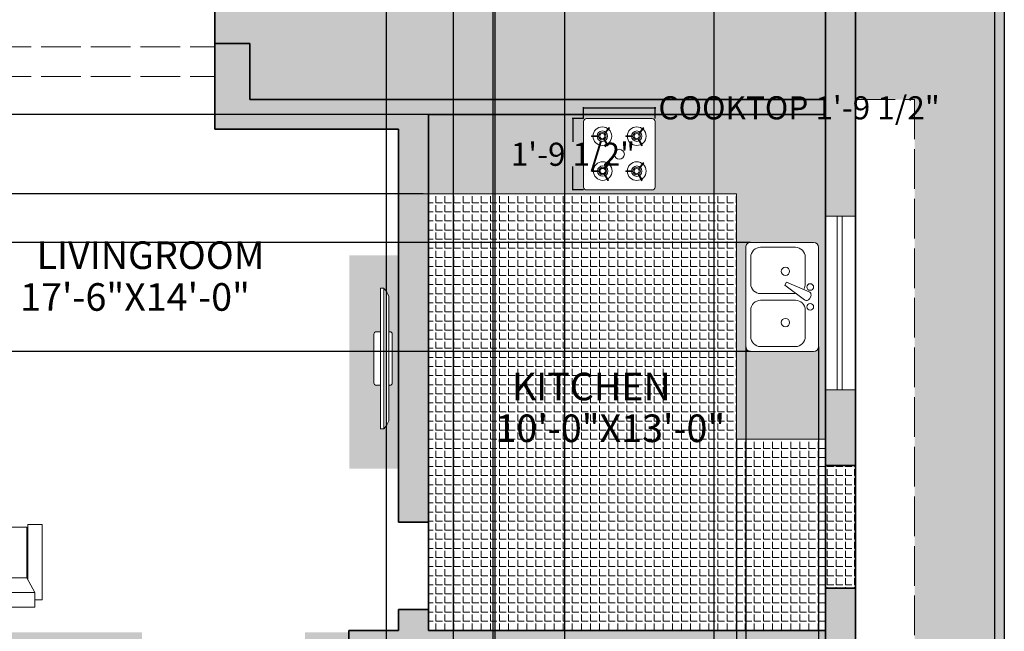
# Model space of a CAD drawing. Units: inches. Extents: x 1884 to 2398, y 474 to 1488.
# Tile 34 of 39: x 2099 to 2397, y 902 to 1087. Entities that reach past the tile are written whole.
import ezdxf

# ---------------------------------------------------------------- set-up
doc = ezdxf.new("R2010")
doc.units = ezdxf.units.IN
doc.header["$MEASUREMENT"] = 0
doc.linetypes.add('ACAD_ISO02W100', pattern=[15, 12, -3])
doc.layers.get('0').update_dxf_attribs({"color": 250})
for name, color, linetype, lineweight in [('A-ANNO-DIMS', 2, 'Continuous', 18), ('A-AREA-IDEN', 7, 'Continuous', 18), ('A-EQPM', 8, 'Continuous', 18), ('A-FLOR-CASE', 8, 'Continuous', 20), ('A-FLOR-FIXT', 8, 'Continuous', 18), ('A-FLOR-OVHD', 8, 'ACAD_ISO02W100', 18), ('A-FLOR-PATT', 254, 'Continuous', 13), ('A-WALL-PATT', 250, 'Continuous', 13), ('C-PROP', 7, 'Continuous', 30), ('furniture', 8, 'Continuous', 18), ('walls', 7, 'Continuous', 35), ('windows', 4, 'Continuous', 18)]:
    doc.layers.add(name, color=color, linetype=linetype, lineweight=lineweight)
doc.layers.add('A-FLOR-CASE-PATT', color=251, linetype='Continuous', lineweight=13, true_color=0x636466)
doc.layers.add('L-PVMT-PATT', color=9, linetype='Continuous', lineweight=13, true_color=0xc7c8ca)
doc.styles.add('ATT', font='TXT')
doc.styles.get("Standard").update_dxf_attribs({"font": 'arial.ttf'})
doc.dimstyles.get("Standard").update_dxf_attribs({"dimtxt": 7, "dimasz": 0.18, "dimexe": 0.18, "dimexo": 0.0625, "dimgap": 0.09, "dimtad": 0, "dimtih": 1, "dimtoh": 1, "dimzin": 0, "dimdsep": 46, "dimlunit": 3, "dimtxsty": 'Standard', "dimcen": 0.09, "dimadec": 0, "dimazin": 0, "dimtfac": 1, "dimtofl": 0, "dimtmove": 0, "dimatfit": 3, "dimfxl": 1, "dimtolj": 1, "dimtzin": 0, "dimarcsym": 0})

# ---------------------------------------------------------------- blocks, each defined once
blk = doc.blocks.new('15PSNK10')
at = {"color": 0, "linetype": 'ByBlock'}
for p, q in [((0, 15), (0, -15)), ((20.5, 16.5), (1.5, 16.5)), ((7, 15), (17.5, 15)), ((22, -15), (22, 15)), ((4, 4), (4, 12)), ((20.5, 12), (20.5, 4)), ((2.37, -0.1), (2.77, 0.6)), ((10.18, -3.57), (4.27, 0.87)), ((17.5, 1), (7, 1)), ((2.88, -1.54), (9.68, -4.43)), ((7.04, -1), (17.5, -1)), ((4, -12), (4, -4)), ((9.68, -4.43), (10.18, -3.57)), ((20.5, -4), (20.5, -12)), ((1.5, -16.5), (20.5, -16.5)), ((17.5, -15), (7, -15))]:
    blk.add_line(p, q, dxfattribs=at)
for centre, radius in [((10, 7.75), 1.25), ((2.5, 3), 1), ((2.5, -3), 1), ((10, -7.75), 1.25)]:
    blk.add_circle(centre, radius, dxfattribs=at)
for centre, radius, start, end in [((1.5, 15), 1.5, 90, 180), ((7, 12), 3, 90, 180), ((17.5, 12), 3, 0, 90), ((20.5, 15), 1.5, 0, 90), ((7, 4), 3, 180, 270), ((17.5, 4), 3, 270, 0), ((3.63, 0.1), 1, 50.5377, 150), ((3.23, -0.6), 1, 150, 249.4623), ((7, -4), 3, 146.607, 180), ((17.5, -4), 3, 0, 90), ((7, -12), 3, 180, 270), ((17.5, -12), 3, 270, 0), ((1.5, -15), 1.5, 180, 270), ((20.5, -15), 1.5, 270, 0)]:
    blk.add_arc(centre, radius, start, end, dxfattribs=at)
at = {"color": 0, "linetype": 'ByBlock', "style": 'ATT'}
for tag, p, flags in [('ITEM', (0, -26), 3), ('ROOM_NUMBER', (0, -35), 1)]:
    blk.add_attdef(tag, p, '', height=6, dxfattribs=dict(at, flags=flags))
blk = doc.blocks.new('4bstove')
at = {"layer": 'furniture'}
for p, q in [((1452.73, 1446.21), (1452.73, 1448.61)), ((1452.98, 1446.22), (1452.98, 1448.61)), ((1464.44, 1446.34), (1464.44, 1448.73)), ((1464.69, 1446.34), (1464.69, 1448.73)), ((1463.45, 1444.58), (1461.38, 1443.38)), ((1451.74, 1444.45), (1449.67, 1443.25)), ((1451.87, 1444.23), (1449.79, 1443.04)), ((1453.75, 1444.08), (1455.58, 1442.54)), ((1453.91, 1444.27), (1455.74, 1442.73)), ((1463.57, 1444.36), (1461.5, 1443.17)), ((1465.46, 1444.21), (1467.29, 1442.67)), ((1465.62, 1444.4), (1467.45, 1442.86)), ((1452.69, 1434.81), (1452.69, 1437.2)), ((1452.94, 1434.81), (1452.94, 1437.2)), ((1464.44, 1434.81), (1464.44, 1437.2)), ((1464.69, 1434.81), (1464.69, 1437.2)), ((1451.7, 1433.04), (1449.63, 1431.85)), ((1451.82, 1432.83), (1449.75, 1431.63)), ((1453.71, 1432.67), (1455.54, 1431.13)), ((1453.87, 1432.86), (1455.7, 1431.33)), ((1463.45, 1433.04), (1461.38, 1431.85)), ((1463.57, 1432.83), (1461.5, 1431.63)), ((1465.46, 1432.67), (1467.29, 1431.13)), ((1465.62, 1432.86), (1467.45, 1431.33))]:
    blk.add_line(p, q, dxfattribs=at)
for points in [[(1447.5, 1427.38), (1469.5, 1427.38, 0.414214), (1470.5, 1428.38), (1470.5, 1450.38, 0.414214), (1469.5, 1451.38), (1447.5, 1451.38, 0.414214), (1446.5, 1450.38), (1446.5, 1428.38, 0.414214)], [(1453.75, 1444.97, 1), (1452, 1444.97, 1)], [(1465.46, 1445.1, 1), (1463.71, 1445.1, 1)], [(1453.71, 1433.56, 1), (1451.96, 1433.56, 1)], [(1465.46, 1433.56, 1), (1463.71, 1433.56, 1)]]:
    blk.add_lwpolyline(points, format="xyb", close=True, dxfattribs=at)
for points in [[(1454.12, 1444.97, 1), (1451.62, 1444.97, 1), (1454.12, 1444.97, 1)], [(1465.83, 1445.1, 1), (1463.33, 1445.1, 1), (1465.83, 1445.1, 1)], [(1454.08, 1433.56, 1), (1451.58, 1433.56, 1), (1454.08, 1433.56, 1)], [(1465.83, 1433.56, 1), (1463.33, 1433.56, 1), (1465.83, 1433.56, 1)]]:
    blk.add_lwpolyline(points, format="xyb", dxfattribs=at)
for centre, radius in [((1452.87, 1444.97), 3.14), ((1464.58, 1445.1), 3.14), ((1452.87, 1444.97), 1.75), ((1464.58, 1445.1), 1.75), ((1458.5, 1439.38), 1.67), ((1452.83, 1433.56), 3.14), ((1452.83, 1433.56), 1.75), ((1464.58, 1433.56), 3.14), ((1464.58, 1433.56), 1.75)]:
    blk.add_circle(centre, radius, dxfattribs=at)
for centre, start, end in [((1452.87, 1444.97), 88.2645, 92.2039), ((1464.58, 1445.1), 88.2645, 92.2039), ((1452.87, 1444.97), 208.188, 212.1274), ((1452.87, 1444.97), 318.1018, 322.0412), ((1464.58, 1445.1), 208.188, 212.1274), ((1464.58, 1445.1), 318.1018, 322.0412), ((1452.83, 1433.56), 88.2645, 92.2039), ((1464.58, 1433.56), 88.2645, 92.2039)]:
    blk.add_arc(centre, 3.64, start, end, dxfattribs=at)
blk = doc.blocks.new('stove')
at = {"layer": 'furniture', "xscale": 0.9, "yscale": 0.9, "zscale": 0.9, "rotation": 89.99999999999999}
blk.add_blockref('4bstove', (1295.44, -1312.65), dxfattribs=at)
blk = doc.blocks.new('PLASMA-LARGE')
at = {"layer": 'furniture'}
for p, q in [((-7.26, 0), (7.26, 0)), ((-21, -2.5), (21, -2.5)), ((-21, -2.5), (-21, -3.5)), ((-18.61, -1), (18.61, -1)), ((-8, -1), (-8, -0.74)), ((8, -1), (8, -0.74)), ((21, -2.5), (21, -3.5)), ((-21, -3.5), (21, -3.5)), ((-8, -3.5), (-8, -4.76)), ((-7.26, -5.5), (7.26, -5.5)), ((8, -3.5), (8, -4.76))]:
    blk.add_line(p, q, dxfattribs=at)
for centre, radius, start, end in [((-7.26, -0.74), 0.744, 90, 180), ((7.26, -0.74), 0.744, 0, 90), ((-13.97, -11.05), 11.07, 114.7602, 129.4175), ((13.97, -11.05), 11.07, 50.5825, 65.2398), ((-7.26, -4.76), 0.744, 180, 270), ((7.26, -4.76), 0.744, 270, 0)]:
    blk.add_arc(centre, radius, start, end, dxfattribs=at)
blk = doc.blocks.new('FABRIC SOFA 1S')
at = {"layer": 'furniture'}
for p, q in [((3, 18.12), (34, 18.12)), ((3, 15.12), (3, 18.12)), ((34, 12.12), (34, 18.12)), ((0, -15.12), (0, 15.12)), ((6, 15.12), (0, 15.12)), ((6, -15.12), (6, 15.12)), ((12, 11.75), (6, 15.12)), ((11.33, 12.12), (34, 12.12)), ((6, -15.12), (12, -11.75)), ((11.33, -12.12), (34, -12.12)), ((34, -12.12), (34, -18.12)), ((6, -15.12), (0, -15.12)), ((3, -18.12), (3, -15.12)), ((3, -18.12), (34, -18.12))]:
    blk.add_line(p, q, dxfattribs=at)
blk.add_lwpolyline([(12, -11.75), (12, 11.75), (33, 11.75), (33, -11.75)], close=True, dxfattribs=at)
blk = doc.blocks.new('*D39')
at = {"layer": 'A-ANNO-DIMS', "color": 0, "lineweight": -2, "transparency": 16777216}
for p, q in [((2269.43, 1056.78), (2269.43, 1060.14)), ((2269.61, 1059.96), (2290.85, 1059.96)), ((2291.03, 1056.78), (2291.03, 1060.14)), ((2291.03, 1059.96), (2291.21, 1059.96))]:
    blk.add_line(p, q, dxfattribs=at)
at = {"layer": 'A-ANNO-DIMS', "color": 0, "lineweight": 100, "transparency": 16777216}
for points in [[(2269.61, 1059.99), (2269.61, 1059.93), (2269.43, 1059.96)], [(2290.85, 1059.99), (2290.85, 1059.93), (2291.03, 1059.96)]]:
    blk.add_solid(points, dxfattribs=at)
at = {"layer": 'Defpoints', "color": 0, "lineweight": 100, "transparency": 16777216}
for p in [(2291.03, 1059.96), (2269.43, 1056.72), (2291.03, 1056.72)]:
    blk.add_point(p, dxfattribs=at)
at = {"layer": 'A-ANNO-DIMS', "color": 0, "transparency": 16777216, "insert": (2334.53, 1059.96), "char_height": 7, "attachment_point": 5}
blk.add_mtext('\\A1;COOKTOP 1\'-9 1/2"', dxfattribs=at)
blk = doc.blocks.new('*D40')
at = {"layer": 'A-ANNO-DIMS', "color": 0, "lineweight": -2, "transparency": 16777216}
for p, q in [((2269.37, 1056.72), (2266.01, 1056.72)), ((2266.19, 1056.54), (2266.19, 1049.63)), ((2266.19, 1035.3), (2266.19, 1042.21)), ((2269.37, 1035.12), (2266.01, 1035.12))]:
    blk.add_line(p, q, dxfattribs=at)
at = {"layer": 'A-ANNO-DIMS', "color": 0, "lineweight": 100, "transparency": 16777216}
for points in [[(2266.16, 1056.54), (2266.22, 1056.54), (2266.19, 1056.72)], [(2266.16, 1035.3), (2266.22, 1035.3), (2266.19, 1035.12)]]:
    blk.add_solid(points, dxfattribs=at)
at = {"layer": 'Defpoints', "color": 0, "lineweight": 100, "transparency": 16777216}
for p in [(2266.19, 1056.72), (2269.43, 1056.72), (2269.43, 1035.12)]:
    blk.add_point(p, dxfattribs=at)
at = {"layer": 'A-ANNO-DIMS', "color": 0, "transparency": 16777216, "insert": (2266.19, 1045.92), "char_height": 7, "attachment_point": 5}
blk.add_mtext('\\A1;1\'-9 1/2"', dxfattribs=at)
blk = doc.blocks.new('*D44')
at = {"layer": 'A-ANNO-DIMS', "color": 0, "lineweight": -2, "transparency": 16777216}
for p, q in [((2209.76, 1247.82), (2209.76, 484)), ((2230.03, 1247.82), (2230.03, 484)), ((2209.94, 484.18), (2229.85, 484.18)), ((2230.03, 484.18), (2230.21, 484.18))]:
    blk.add_line(p, q, dxfattribs=at)
at = {"layer": 'A-ANNO-DIMS', "color": 0, "lineweight": 100, "transparency": 16777216}
for points in [[(2209.94, 484.21), (2209.94, 484.15), (2209.76, 484.18)], [(2229.85, 484.21), (2229.85, 484.15), (2230.03, 484.18)]]:
    blk.add_solid(points, dxfattribs=at)
at = {"layer": 'Defpoints', "color": 0, "lineweight": 100, "transparency": 16777216}
for p in [(2209.76, 1247.88), (2230.03, 1247.88), (2230.03, 484.18)]:
    blk.add_point(p, dxfattribs=at)
at = {"layer": 'A-ANNO-DIMS', "color": 0, "transparency": 16777216, "insert": (2247.43, 484.18), "char_height": 7, "attachment_point": 5}
blk.add_mtext('\\A1;1\'-8 1/2"', dxfattribs=at)
blk = doc.blocks.new('*D45')
at = {"layer": 'A-ANNO-DIMS', "color": 0, "lineweight": -2, "transparency": 16777216}
for p, q in [((2242.62, 1322.82), (2242.62, 484)), ((2263.62, 1322.82), (2263.62, 484)), ((2242.8, 484.18), (2244.05, 484.18)), ((2263.44, 484.18), (2262.18, 484.18))]:
    blk.add_line(p, q, dxfattribs=at)
at = {"layer": 'A-ANNO-DIMS', "color": 0, "lineweight": 100, "transparency": 16777216}
for points in [[(2242.8, 484.21), (2242.8, 484.15), (2242.62, 484.18)], [(2263.44, 484.21), (2263.44, 484.15), (2263.62, 484.18)]]:
    blk.add_solid(points, dxfattribs=at)
at = {"layer": 'Defpoints', "color": 0, "lineweight": 100, "transparency": 16777216}
for p in [(2242.62, 1322.88), (2263.62, 1322.88), (2263.62, 484.18)]:
    blk.add_point(p, dxfattribs=at)
at = {"layer": 'A-ANNO-DIMS', "color": 0, "transparency": 16777216, "insert": (2253.12, 484.18), "char_height": 7, "attachment_point": 5}
blk.add_mtext('\\A1;1\'-9"', dxfattribs=at)
blk = doc.blocks.new('*D47')
at = {"layer": 'A-ANNO-DIMS', "color": 0, "lineweight": -2, "transparency": 16777216}
for p, q in [((2315.59, 959.7), (2315.59, 484)), ((2342.53, 959.7), (2342.53, 484)), ((2315.77, 484.18), (2319.61, 484.18)), ((2342.35, 484.18), (2338.51, 484.18))]:
    blk.add_line(p, q, dxfattribs=at)
at = {"layer": 'A-ANNO-DIMS', "color": 0, "lineweight": 100, "transparency": 16777216}
for points in [[(2315.77, 484.21), (2315.77, 484.15), (2315.59, 484.18)], [(2342.35, 484.21), (2342.35, 484.15), (2342.53, 484.18)]]:
    blk.add_solid(points, dxfattribs=at)
at = {"layer": 'Defpoints', "color": 0, "lineweight": 100, "transparency": 16777216}
for p in [(2315.59, 959.77), (2342.53, 959.77), (2342.53, 484.18)]:
    blk.add_point(p, dxfattribs=at)
at = {"layer": 'A-ANNO-DIMS', "color": 0, "transparency": 16777216, "insert": (2329.06, 484.18), "char_height": 7, "attachment_point": 5}
blk.add_mtext('\\A1;2\'-3"', dxfattribs=at)
blk = doc.blocks.new('*D48')
at = {"layer": 'A-ANNO-DIMS', "color": 0, "lineweight": -2, "transparency": 16777216}
for p, q in [((2222.47, 1057.97), (1902.43, 1057.97)), ((1902.61, 1057.79), (1902.61, 1049.64)), ((1902.61, 1034.16), (1902.61, 1042.31)), ((2220.98, 1033.98), (1902.43, 1033.98))]:
    blk.add_line(p, q, dxfattribs=at)
at = {"layer": 'A-ANNO-DIMS', "color": 0, "lineweight": 100, "transparency": 16777216}
for points in [[(1902.58, 1057.79), (1902.64, 1057.79), (1902.61, 1057.97)], [(1902.58, 1034.16), (1902.64, 1034.16), (1902.61, 1033.98)]]:
    blk.add_solid(points, dxfattribs=at)
at = {"layer": 'Defpoints', "color": 0, "lineweight": 100, "transparency": 16777216}
for p in [(1902.61, 1057.97), (2222.53, 1057.97), (2221.05, 1033.98)]:
    blk.add_point(p, dxfattribs=at)
at = {"layer": 'A-ANNO-DIMS', "color": 0, "transparency": 16777216, "insert": (1902.61, 1045.97), "char_height": 7, "attachment_point": 5}
blk.add_mtext('\\A1;2\'-0"', dxfattribs=at)
blk = doc.blocks.new('*D49')
at = {"layer": 'A-ANNO-DIMS', "color": 0, "lineweight": -2, "transparency": 16777216}
for p, q in [((2318.41, 987.72), (2318.41, 484)), ((2340.41, 987.72), (2340.41, 484)), ((2318.59, 484.18), (2340.23, 484.18)), ((2340.41, 484.18), (2340.59, 484.18))]:
    blk.add_line(p, q, dxfattribs=at)
at = {"layer": 'A-ANNO-DIMS', "color": 0, "lineweight": 100, "transparency": 16777216}
for points in [[(2318.59, 484.21), (2318.59, 484.15), (2318.41, 484.18)], [(2340.23, 484.21), (2340.23, 484.15), (2340.41, 484.18)]]:
    blk.add_solid(points, dxfattribs=at)
at = {"layer": 'Defpoints', "color": 0, "lineweight": 100, "transparency": 16777216}
for p in [(2318.41, 987.78), (2340.41, 987.78), (2340.41, 484.18)]:
    blk.add_point(p, dxfattribs=at)
at = {"layer": 'A-ANNO-DIMS', "color": 0, "transparency": 16777216, "insert": (2352.37, 484.18), "char_height": 7, "attachment_point": 5}
blk.add_mtext('\\A1;1\'-10"', dxfattribs=at)
blk = doc.blocks.new('*D50')
at = {"layer": 'A-ANNO-DIMS', "color": 0, "lineweight": -2, "transparency": 16777216}
for p, q in [((2319.85, 1019.28), (1902.43, 1019.28)), ((1902.61, 1019.1), (1902.61, 1006.44)), ((1902.61, 986.46), (1902.61, 999.11)), ((2319.85, 986.28), (1902.43, 986.28))]:
    blk.add_line(p, q, dxfattribs=at)
at = {"layer": 'A-ANNO-DIMS', "color": 0, "lineweight": 100, "transparency": 16777216}
for points in [[(1902.58, 1019.1), (1902.64, 1019.1), (1902.61, 1019.28)], [(1902.58, 986.46), (1902.64, 986.46), (1902.61, 986.28)]]:
    blk.add_solid(points, dxfattribs=at)
at = {"layer": 'Defpoints', "color": 0, "lineweight": 100, "transparency": 16777216}
for p in [(1902.61, 1019.28), (2319.91, 1019.28), (2319.91, 986.28)]:
    blk.add_point(p, dxfattribs=at)
at = {"layer": 'A-ANNO-DIMS', "color": 0, "transparency": 16777216, "insert": (1902.61, 1002.78), "char_height": 7, "attachment_point": 5}
blk.add_mtext('\\A1;2\'-9"', dxfattribs=at)
blk = doc.blocks.new('*D52')
at = {"layer": 'A-ANNO-DIMS', "color": 0, "lineweight": -2, "transparency": 16777216}
for p, q in [((2308.85, 820.89), (2308.85, 1477.76)), ((2309.03, 1477.58), (2342.35, 1477.58)), ((2342.53, 820.89), (2342.53, 1477.76)), ((2342.53, 1477.58), (2342.71, 1477.58))]:
    blk.add_line(p, q, dxfattribs=at)
at = {"layer": 'A-ANNO-DIMS', "color": 0, "lineweight": 100, "transparency": 16777216}
for points in [[(2309.03, 1477.61), (2309.03, 1477.55), (2308.85, 1477.58)], [(2342.35, 1477.61), (2342.35, 1477.55), (2342.53, 1477.58)]]:
    blk.add_solid(points, dxfattribs=at)
at = {"layer": 'Defpoints', "color": 0, "lineweight": 100, "transparency": 16777216}
for p in [(2342.53, 1477.58), (2308.85, 820.83), (2342.53, 820.83)]:
    blk.add_point(p, dxfattribs=at)
at = {"layer": 'A-ANNO-DIMS', "color": 0, "transparency": 16777216, "insert": (2360.32, 1477.58), "char_height": 7, "attachment_point": 5}
blk.add_mtext('\\A1;2\'-9 1/2"', dxfattribs=at)
blk = doc.blocks.new('*D54')
at = {"layer": 'A-ANNO-DIMS', "color": 0, "lineweight": -2, "transparency": 16777216}
for p, q in [((2242.06, 893.03), (2242.06, 1477.76)), ((2242.24, 1477.58), (2266.06, 1477.58)), ((2308.67, 1477.58), (2284.85, 1477.58)), ((2308.85, 893.03), (2308.85, 1477.76))]:
    blk.add_line(p, q, dxfattribs=at)
at = {"layer": 'A-ANNO-DIMS', "color": 0, "lineweight": 100, "transparency": 16777216}
for points in [[(2242.24, 1477.61), (2242.24, 1477.55), (2242.06, 1477.58)], [(2308.67, 1477.61), (2308.67, 1477.55), (2308.85, 1477.58)]]:
    blk.add_solid(points, dxfattribs=at)
at = {"layer": 'Defpoints', "color": 0, "lineweight": 100, "transparency": 16777216}
for p in [(2308.85, 1477.58), (2242.06, 892.97), (2308.85, 892.97)]:
    blk.add_point(p, dxfattribs=at)
at = {"layer": 'A-ANNO-DIMS', "color": 0, "transparency": 16777216, "insert": (2275.45, 1477.58), "char_height": 7, "attachment_point": 5}
blk.add_mtext('\\A1;5\'-7"', dxfattribs=at)

msp = doc.modelspace()

# ---------------------------------------------------------------- hatches: boundary and pattern name
at = {"layer": 'A-FLOR-CASE-PATT'}
h = msp.add_hatch(color=256, dxfattribs=at)
h.dxf.hatch_style = 1
h.paths.add_polyline_path([(2342.529, 1057.966), (2222.529, 1057.966), (2222.529, 1033.976), (2315.591, 1033.976), (2315.591, 959.766), (2342.529, 959.766)])
h.paths.add_polyline_path([(2269.433, 1055.817, -0.4142136), (2270.333, 1056.717), (2290.133, 1056.717, -0.4142136), (2291.033, 1055.817), (2291.033, 1036.017, -0.4142136), (2290.133, 1035.117), (2270.333, 1035.117, -0.4142136), (2269.433, 1036.017)], flags=16)
h.paths.add_polyline_path([(2271.815, 1051.262, -0.0171907), (2271.814, 1051.487), (2272.265, 1051.487, -0.6105283), (2276.81, 1053.623), (2277.099, 1053.968, -0.0171906), (2277.272, 1053.824), (2276.982, 1053.479, -0.2116406), (2277.909, 1051.388, -0.2564461), (2276.601, 1049.006), (2276.827, 1048.616, -0.0171907), (2276.632, 1048.503), (2276.407, 1048.893, -0.5505708), (2272.266, 1051.262)], flags=0)
h.paths.add_polyline_path([(2271.929, 1040.951), (2272.379, 1040.951, -0.6105283), (2276.925, 1043.087), (2277.214, 1043.432, -0.0171906), (2277.387, 1043.288), (2277.097, 1042.943, -0.2116406), (2278.024, 1040.852, -0.2564461), (2276.716, 1038.47), (2276.941, 1038.08, -0.0171907), (2276.747, 1037.967), (2276.522, 1038.357, -0.5505708), (2272.38, 1040.726), (2271.93, 1040.726, -0.0171907)], flags=0)
h.paths.add_polyline_path([(2276.661, 1051.388, -1), (2273.511, 1051.388, -1)], flags=0)
h.paths.add_polyline_path([(2275.086, 1052.513, -1), (2275.086, 1050.263, -1)], flags=0)
h.paths.add_polyline_path([(2275.086, 1052.175, -1), (2275.086, 1050.6, -1)], flags=0)
h.paths.add_polyline_path([(2276.776, 1040.852, -1), (2273.626, 1040.852, -1)], flags=0)
h.paths.add_polyline_path([(2275.201, 1041.977, -1), (2275.201, 1039.727, -1)], flags=0)
h.paths.add_polyline_path([(2275.201, 1041.639, -1), (2275.201, 1040.064, -1)], flags=0)
h.paths.add_polyline_path([(2281.737, 1045.917, -1), (2278.73, 1045.917, -1)], flags=0)
h.paths.add_polyline_path([(2282.197, 1051.262, -0.0171907), (2282.196, 1051.487), (2282.647, 1051.487, -0.9825922), (2288.291, 1051.388, -0.9779445), (2282.648, 1051.262)], flags=0)
h.paths.add_polyline_path([(2282.196, 1040.912), (2282.647, 1040.912, -0.9825922), (2288.291, 1040.813, -0.9779445), (2282.648, 1040.687), (2282.197, 1040.687, -0.0171907)], flags=0)
h.paths.add_polyline_path([(2287.043, 1051.388, -1), (2283.893, 1051.388, -1)], flags=0)
h.paths.add_polyline_path([(2285.468, 1052.513, -1), (2285.468, 1050.263, -1)], flags=0)
h.paths.add_polyline_path([(2285.468, 1052.175, -1), (2285.468, 1050.6, -1)], flags=0)
h.paths.add_polyline_path([(2287.043, 1040.813, -1), (2283.893, 1040.813, -1)], flags=0)
h.paths.add_polyline_path([(2285.468, 1041.938, -1), (2285.468, 1039.688, -1)], flags=0)
h.paths.add_polyline_path([(2285.468, 1041.601, -1), (2285.468, 1040.026, -1)], flags=0)
h.paths.add_polyline_path([(2319.909, 1019.278), (2338.909, 1019.278, -0.4142136), (2340.409, 1017.778), (2340.409, 987.778, -0.4142136), (2338.909, 986.278), (2319.909, 986.278, -0.4142136), (2318.409, 987.778), (2318.409, 1017.778, -0.4142136)], flags=16)
h.paths.add_polyline_path([(2337.528, 1004.314, -0.4631995), (2338.044, 1002.878), (2337.641, 1002.18, -0.4369422), (2336.21, 1001.854), (2330.231, 1006.345), (2330.731, 1007.211)], flags=0)
h.paths.add_polyline_path([(2322.909, 1001.778), (2333.409, 1001.778, -0.4142136), (2336.409, 998.778), (2336.409, 990.778, -0.4142136), (2333.409, 987.778), (2322.909, 987.778, -0.4142136), (2319.909, 990.778), (2319.909, 998.778, -0.4142136)], flags=0)
h.paths.add_polyline_path([(2331.659, 1010.528, -1), (2329.159, 1010.528, -1)], flags=0)
h.paths.add_polyline_path([(2331.659, 995.028, -1), (2329.159, 995.028, -1)], flags=0)
h.paths.add_polyline_path([(2338.909, 1005.778, -1), (2336.909, 1005.778, -1)], flags=0)
h.paths.add_polyline_path([(2338.909, 999.778, -1), (2336.909, 999.778, -1)], flags=0)
h = msp.add_hatch(color=256, dxfattribs=at)
h.dxf.hatch_style = 1
h.paths.add_polyline_path([(2198.68, 1015.326), (2213.576, 1015.326), (2213.576, 950.883), (2198.68, 950.883)])
h.paths.add_polyline_path([(2208.087, 962.907), (2209.098, 962.907, 0.0640419), (2210.615, 965.326), (2210.615, 976.054), (2210.874, 976.054, 0.4142136), (2211.626, 976.807), (2211.626, 991.482, 0.4142136), (2210.874, 992.235), (2210.615, 992.235), (2210.615, 1002.962, 0.0640419), (2209.098, 1005.381), (2208.087, 1005.381), (2208.087, 992.235), (2206.817, 992.235, 0.4142136), (2206.064, 991.482), (2206.064, 976.807, 0.4142136), (2206.817, 976.054), (2208.087, 976.054)], flags=16)
at = {"layer": 'A-FLOR-PATT'}
h = msp.add_hatch(color=256, dxfattribs=at)
h.dxf.hatch_style = 1
h.paths.add_polyline_path([(2117.529, 815.801), (2126.529, 815.801), (2126.529, 880.382), (2117.529, 880.382), (2117.529, 892.385), (1961.529, 892.385), (1961.529, 756.915), (1964.529, 756.915), (1964.529, 759.915), (1995.529, 759.915), (1995.529, 753.915), (1972.862, 753.915), (1967.529, 756.915), (1967.529, 654.915), (1972.862, 657.915), (1995.529, 657.915), (1995.529, 651.915), (1964.529, 651.915), (1964.529, 654.915), (1961.529, 654.915), (1961.529, 640.385), (2117.529, 640.385), (2117.529, 646.578), (2126.529, 646.578), (2126.529, 676.183), (2117.529, 676.183)])
h.paths.add_polyline_path([(2012.246, 808.929), (2012.05, 810.185), (2032.542, 810.185), (2032.346, 808.929)], flags=16)
h.paths.add_polyline_path([(2010.381, 820.864), (1994.658, 820.864), (1994.658, 831.561), (1984.608, 833.132), (1984.608, 853.821), (1994.658, 855.391), (1994.658, 866.089), (2010.381, 866.089), (2011.951, 876.139), (2032.64, 876.139), (2034.211, 866.089), (2045.556, 866.089), (2047.127, 876.139), (2067.816, 876.139), (2069.386, 866.089), (2085.109, 866.089), (2085.109, 855.391), (2095.159, 853.821), (2095.159, 833.132), (2085.109, 831.561), (2085.109, 820.864), (2069.386, 820.864), (2067.816, 810.814), (2047.127, 810.814), (2045.556, 820.864), (2034.211, 820.864), (2032.64, 810.814), (2011.951, 810.814)], flags=16)
h.paths.add_polyline_path([(1982.724, 833.426), (1982.724, 853.526), (1983.98, 853.723), (1983.98, 833.23)], flags=16)
h.paths.add_polyline_path([(1994.529, 753.54), (1994.529, 658.29), (1973.529, 658.29), (1973.529, 753.54)], flags=16)
h.paths.add_polyline_path([(2084.486, 843.527), (2084.592, 843.502), (2084.681, 843.487), (2084.813, 843.477), (2084.913, 843.477), (2084.669, 843.482), (2084.336, 843.565), (2084.116, 843.617), (2083.8, 843.686), (2083.105, 843.827), (2082.836, 843.874), (2083.604, 843.729), (2084.206, 843.597)], flags=0)
h.paths.add_polyline_path([(2047.421, 808.929), (2047.225, 810.185), (2067.718, 810.185), (2067.521, 808.929)], flags=16)
h.paths.add_polyline_path([(2066.01, 849.505), (2066.429, 849.687), (2066.798, 849.882), (2067.129, 850.085), (2067.43, 850.293), (2067.711, 850.502), (2068.176, 850.856), (2068.689, 851.205), (2069.305, 851.531), (2070.015, 851.784), (2070.844, 851.944), (2071.081, 851.956), (2070.629, 851.902), (2070.212, 851.822), (2069.827, 851.717), (2069.471, 851.59), (2069.139, 851.443), (2068.828, 851.279), (2068.534, 851.1), (2068.254, 850.909), (2067.983, 850.709), (2067.502, 850.343), (2066.951, 849.962), (2066.224, 849.579)], flags=0)
h.paths.add_polyline_path([(2059.423, 853.221), (2059.827, 853.278), (2060.171, 853.358), (2060.465, 853.463), (2060.714, 853.589), (2060.926, 853.736), (2061.107, 853.902), (2061.258, 854.086), (2061.377, 854.284), (2061.462, 854.495), (2061.514, 854.715), (2061.53, 854.943), (2061.508, 855.176), (2061.449, 855.411), (2061.352, 855.646), (2061.224, 855.882), (2061.07, 856.117), (2060.9, 856.353), (2060.719, 856.588), (2060.406, 856.993), (2060.103, 857.424), (2059.858, 857.888), (2059.691, 858.467), (2059.836, 859.091), (2060.305, 859.532), (2060.844, 859.798), (2061.513, 859.935), (2062.253, 859.905), (2062.483, 859.849), (2062.078, 859.912), (2061.695, 859.928), (2061.336, 859.899), (2061.005, 859.831), (2060.703, 859.729), (2060.437, 859.597), (2060.208, 859.441), (2060.021, 859.265), (2059.879, 859.075), (2059.785, 858.874), (2059.737, 858.664), (2059.73, 858.447), (2059.761, 858.224), (2059.827, 857.996), (2059.923, 857.765), (2060.047, 857.53), (2060.193, 857.295), (2060.359, 857.06), (2060.537, 856.824), (2060.867, 856.399), (2061.171, 855.978), (2061.422, 855.518), (2061.567, 854.943), (2061.41, 854.272), (2060.947, 853.707), (2060.335, 853.397), (2059.649, 853.236)], flags=0)
h.paths.add_polyline_path([(2050.778, 859.745), (2051.07, 859.87), (2051.295, 860.017), (2051.467, 860.183), (2051.594, 860.365), (2051.679, 860.56), (2051.726, 860.763), (2051.739, 860.971), (2051.722, 861.18), (2051.677, 861.387), (2051.609, 861.587), (2051.521, 861.779), (2051.421, 861.962), (2051.312, 862.138), (2051.203, 862.307), (2050.966, 862.68), (2050.793, 863.193), (2051.021, 863.699), (2051.483, 864.018), (2052.09, 864.138), (2052.773, 864.157), (2053.007, 864.142), (2052.603, 864.152), (2052.258, 864.142), (2051.965, 864.113), (2051.716, 864.064), (2051.504, 863.995), (2051.322, 863.907), (2051.17, 863.802), (2051.048, 863.682), (2050.954, 863.55), (2050.891, 863.408), (2050.856, 863.259), (2050.851, 863.105), (2050.876, 862.948), (2050.929, 862.791), (2051.005, 862.633), (2051.098, 862.472), (2051.203, 862.307), (2051.312, 862.138), (2051.556, 861.742), (2051.751, 861.167), (2051.712, 860.535), (2051.398, 860.085), (2050.949, 859.79)], flags=0)
h.paths.add_polyline_path([(2022.768, 719.264), (2050.461, 719.264), (2050.461, 717.226), (2052.426, 717.226), (2052.426, 715.033), (2050.461, 715.033), (2050.461, 703.738), (2022.768, 703.738)], flags=16)
h.paths.add_polyline_path([(2012.246, 878.023), (2032.346, 878.023), (2032.542, 876.767), (2012.05, 876.767)], flags=16)
h.paths.add_polyline_path([(2035.324, 713.103), (2035.342, 713.294), (2035.192, 713.202)], flags=0)
h.paths.add_polyline_path([(2036.484, 711.63), (2036.583, 711.849), (2036.39, 711.898)], flags=0)
h.paths.add_polyline_path([(2036.074, 712.744), (2035.993, 712.481), (2035.724, 712.516), (2035.794, 712.726)], flags=0)
h.paths.add_polyline_path([(2035.846, 710.909), (2035.753, 710.958), (2035.702, 710.88)], flags=0)
h.paths.add_polyline_path([(2037.818, 712.019), (2037.948, 712.06), (2037.987, 712.161), (2037.815, 712.02)], flags=0)
h.paths.add_polyline_path([(2038.451, 709.517), (2038.464, 709.428), (2038.586, 709.442)], flags=0)
h.paths.add_polyline_path([(2037.805, 709.806), (2037.818, 709.807), (2037.804, 709.823)], flags=0)
h.paths.add_polyline_path([(2036.7, 711.245), (2036.698, 711.236), (2036.813, 711.211)], flags=0)
h.paths.add_polyline_path([(2035.928, 708.897), (2035.668, 708.871), (2035.706, 708.667)], flags=0)
h.paths.add_polyline_path([(2036.414, 710.976), (2035.932, 709.859), (2036.792, 710.484), (2036.5, 710.934)], flags=0)
h.paths.add_polyline_path([(2038.298, 712.115), (2038.499, 712.058), (2038.612, 712.269), (2038.39, 712.332)], flags=0)
h.paths.add_polyline_path([(2047.421, 878.023), (2067.521, 878.023), (2067.718, 876.767), (2047.225, 876.767)], flags=16)
h.paths.add_polyline_path([(2049.647, 705.093, -1), (2048.845, 705.093, -1)], flags=0)
h.paths.add_polyline_path([(2095.787, 853.723), (2097.043, 853.526), (2097.043, 833.426), (2095.787, 833.23)], flags=16)
h.paths.add_polyline_path([(2110.739, 745.339), (2111.75, 745.339, -0.0640419), (2113.267, 742.92), (2113.267, 732.192), (2113.526, 732.192, -0.4142136), (2114.278, 731.439), (2114.278, 716.764, -0.4142136), (2113.526, 716.011), (2113.267, 716.011), (2113.267, 705.284, -0.0640419), (2111.75, 702.864), (2110.739, 702.864), (2110.739, 716.011), (2109.469, 716.011, -0.4142136), (2108.716, 716.764), (2108.716, 731.439, -0.4142136), (2109.469, 732.192), (2110.739, 732.192)], flags=16)
h.paths.add_polyline_path([(1998.045, 668.909), (2002.449, 668.909), (2002.449, 652.273), (2002.724, 652.763), (2002.724, 668.175), (2019.972, 668.175), (2019.972, 652.763), (2020.247, 652.273), (2020.247, 668.909), (2024.651, 668.909), (2029.055, 668.909), (2029.055, 652.273), (2029.33, 652.763), (2029.33, 668.175), (2046.578, 668.175), (2046.578, 652.763), (2046.853, 652.273), (2046.853, 668.909), (2051.257, 668.909), (2051.257, 646.157), (2049.055, 646.157), (2049.055, 643.955), (2026.853, 643.955), (2026.853, 646.157), (2024.651, 646.157), (2022.449, 646.157), (2022.449, 643.955), (2000.247, 643.955), (2000.247, 646.157), (1998.045, 646.157)], flags=16)
h.paths.add_polyline_path([(2342.529, 1247.885), (2265.892, 1247.885), (2230.029, 1247.885), (2209.755, 1247.885), (2168.6, 1247.885), (2168.6, 1104.929), (2158.029, 1104.929), (2158.029, 1079.411), (2168.6, 1079.411), (2168.6, 1062.466), (2342.529, 1062.466), (2342.529, 1093.809)])
h.paths.add_polyline_path([(2215.03, 1153.876), (2215.03, 1164.739), (2187.559, 1164.739), (2187.442, 1152.641), (2173.568, 1152.641), (2173.684, 1164.739), (2173.684, 1218.739), (2173.801, 1230.837), (2187.675, 1230.837), (2187.559, 1218.739), (2215.03, 1218.739), (2215.03, 1225.879), (2245.053, 1225.879), (2245.053, 1153.876)], flags=16)
h.paths.add_polyline_path([(2192.147, 1164.797), (2184.963, 1174.54), (2184.915, 1174.54), (2176.755, 1174.54), (2176.755, 1190.363), (2184.915, 1190.363), (2184.915, 1196.819), (2176.755, 1196.819), (2176.755, 1212.641), (2184.915, 1212.641), (2184.915, 1174.606), (2184.963, 1174.54), (2192.147, 1174.54)], flags=0)
h.paths.add_polyline_path([(2184.971, 1158.364, -1), (2176.039, 1158.364, -1)], flags=0)
h.paths.add_polyline_path([(2335.555, 1161.985), (2335.555, 1175.132), (2334.285, 1175.132, -0.4142136), (2333.533, 1175.885), (2333.533, 1190.56, -0.4142136), (2334.285, 1191.313), (2335.555, 1191.313), (2335.555, 1204.46), (2336.567, 1204.46, -0.0640419), (2338.083, 1202.04), (2338.083, 1191.313), (2338.342, 1191.313, -0.4142136), (2339.095, 1190.56), (2339.095, 1175.885, -0.4142136), (2338.342, 1175.132), (2338.083, 1175.132), (2338.083, 1164.405, -0.0640419), (2336.567, 1161.985)], flags=16)
h.paths.add_polyline_path([(2176.155, 1224.462, -1), (2185.087, 1224.462, -1)], flags=0)
h.paths.add_polyline_path([(2158.029, 1276.197), (2158.029, 1322.885), (2148.233, 1322.885), (2092.029, 1322.885), (1961.529, 1322.885), (1961.529, 1166.885), (2116.005, 1166.885), (2116.005, 1157.885), (2152.638, 1157.885), (2152.638, 1166.885), (2158.029, 1166.885)])
h.paths.add_polyline_path([(2006.352, 1204.245), (2006.352, 1215.108), (1978.881, 1215.108), (1978.764, 1203.01), (1964.89, 1203.01), (1965.006, 1215.108), (1965.006, 1269.108), (1965.123, 1281.207), (1978.997, 1281.207), (1978.881, 1269.108), (2006.352, 1269.108), (2006.352, 1276.248), (2036.375, 1276.248), (2036.375, 1204.245)], flags=16)
h.paths.add_polyline_path([(1983.469, 1215.166), (1976.285, 1224.909), (1976.237, 1224.909), (1968.077, 1224.909), (1968.077, 1240.732), (1976.237, 1240.732), (1976.237, 1247.188), (1968.077, 1247.188), (1968.077, 1263.011), (1976.237, 1263.011), (1976.237, 1224.975), (1976.285, 1224.909), (1983.469, 1224.909)], flags=0)
h.paths.add_polyline_path([(1976.293, 1208.733, -1), (1967.361, 1208.733, -1)], flags=0)
h.paths.add_polyline_path([(1967.477, 1274.832, -1), (1976.41, 1274.832, -1)], flags=0)
h.paths.add_polyline_path([(2152.587, 1223.485), (2152.587, 1236.632), (2151.317, 1236.632, -0.4142136), (2150.564, 1237.385), (2150.564, 1252.06, -0.4142136), (2151.317, 1252.813), (2152.587, 1252.813), (2152.587, 1265.959), (2153.598, 1265.959, -0.0640419), (2155.115, 1263.54), (2155.115, 1252.813), (2155.374, 1252.813, -0.4142136), (2156.126, 1252.06), (2156.126, 1237.385, -0.4142136), (2155.374, 1236.632), (2155.115, 1236.632), (2155.115, 1225.904, -0.0640419), (2153.598, 1223.485)], flags=16)
h.paths.add_polyline_path([(2250.676, 1161.101), (2322.077, 1161.101), (2322.077, 1173.886), (2250.676, 1173.886)], flags=24)
h.paths.add_polyline_path([(2255.61, 1173.712), (2320.136, 1173.712), (2320.136, 1186.659), (2255.61, 1186.659)], flags=24)
h.paths.add_polyline_path([(2053.687, 1230.837), (2125.089, 1230.837), (2125.089, 1243.622), (2053.687, 1243.622)], flags=24)
h.paths.add_polyline_path([(2058.622, 1243.448), (2123.147, 1243.448), (2123.147, 1256.395), (2058.622, 1256.395)], flags=24)
h = msp.add_hatch(dxfattribs=at)
h.set_pattern_fill('ANGLE', color=256, scale=10)
h.set_pattern_definition([(0, (0, 0), (0, 2.75), [2, -0.75]), (90, (0, 0), (-2.75, 2e-16), [2, -0.75])])
h.paths.add_polyline_path([(2315.591, 1033.976), (2222.529, 1033.976), (2222.529, 934.675), (2222.529, 901.966), (2342.529, 901.966), (2342.529, 914.773), (2351.529, 914.773), (2351.529, 951.86), (2342.529, 951.86), (2342.529, 959.766), (2315.591, 959.766)])
at = {"layer": 'A-WALL-PATT'}
h = msp.add_hatch(color=256, dxfattribs=at)
h.dxf.hatch_style = 1
h.paths.add_polyline_path([(2092.029, 1406.885), (1952.529, 1406.885), (1952.529, 939.249), (1955.529, 939.249), (1955.529, 1069.385), (1969.695, 1069.385), (1969.695, 1078.385), (1961.529, 1078.385), (1961.529, 1397.885), (2087.529, 1397.885), (2087.529, 1322.885), (2092.029, 1322.885), (2092.029, 1328.623)])
h.paths.add_polyline_path([(2087.529, 1345.919), (2014.612, 1345.919), (2014.612, 1327.385), (2007.132, 1327.385), (2007.132, 1322.885), (2019.112, 1322.885), (2019.112, 1327.385), (2019.112, 1341.419), (2087.529, 1341.419)], flags=17)
h.paths.add_polyline_path([(1965.066, 1327.561), (1961.529, 1327.561), (1961.529, 1322.885), (1965.066, 1322.885)], flags=17)
h.paths.add_polyline_path([(2351.529, 1343.885), (2265.892, 1343.885), (2164.726, 1343.885), (2158.029, 1343.885), (2158.029, 1334.885), (2158.029, 1328.623), (2148.233, 1328.623), (2148.233, 1322.885), (2158.029, 1322.885), (2158.029, 1276.197), (2158.029, 1166.885), (2152.638, 1166.885), (2152.638, 1157.885), (2158.029, 1157.885), (2158.029, 1104.929), (2168.6, 1104.929), (2168.6, 1247.885), (2209.755, 1247.885), (2209.755, 1252.385), (2167.029, 1252.385), (2167.029, 1334.885), (2265.892, 1334.885), (2342.529, 1334.885), (2342.529, 1310.041), (2351.529, 1310.041)])
h.paths.add_polyline_path([(2234.529, 1334.885), (2230.029, 1334.885), (2230.029, 1275.554), (2234.529, 1275.554)], flags=17)
h.paths.add_polyline_path([(2342.529, 1252.385), (2265.892, 1252.385), (2234.529, 1252.385), (2234.529, 1256.117), (2230.029, 1256.117), (2230.029, 1247.885), (2265.892, 1247.885), (2342.529, 1247.885)], flags=17)
h.paths.add_polyline_path([(2351.529, 1276.197), (2351.529, 1293.635), (2342.529, 1293.635), (2342.529, 1252.385), (2342.529, 1225.302), (2346.311, 1225.302), (2351.529, 1225.302)], flags=17)
h.paths.add_polyline_path([(2351.529, 1126.264), (2342.529, 1126.264), (2342.529, 1093.809), (2342.529, 1062.466), (2168.6, 1062.466), (2168.6, 1079.411), (2158.029, 1079.411), (2158.029, 1056.803), (2158.029, 1053.466), (2213.529, 1053.466), (2213.529, 934.675), (2222.529, 934.675), (2222.529, 1057.966), (2342.529, 1057.966), (2342.529, 1027.206), (2345.987, 1027.206), (2351.529, 1027.206)])
h.paths.add_polyline_path([(2116.005, 1166.885), (1961.529, 1166.885), (1961.529, 1162.385), (2081.529, 1162.385), (2081.529, 1152.292), (2090.529, 1152.292), (2090.529, 1157.885), (2116.005, 1157.885)])
h.paths.add_polyline_path([(2090.529, 1122.635), (2081.529, 1122.635), (2081.529, 1078.385), (2000.529, 1078.385), (2000.529, 1069.385), (2000.529, 1034.463), (2003.893, 1034.463), (2009.529, 1034.463), (2009.529, 1069.385), (2090.529, 1069.385)], flags=17)
h.paths.add_polyline_path([(2351.529, 974.676), (2342.529, 974.676), (2342.529, 951.86), (2351.529, 951.86)], flags=17)
h = msp.add_hatch(color=256, dxfattribs=at)
h.dxf.hatch_style = 1
h.paths.add_polyline_path([(2396.529, 1406.885), (2393.529, 1406.885), (2393.529, 1061.532), (2396.529, 1061.532)])
h = msp.add_hatch(color=256, dxfattribs=at)
h.dxf.hatch_style = 1
h.paths.add_polyline_path([(2396.529, 1406.885), (2393.529, 1406.885), (2393.529, 779.322), (2396.529, 779.322)])
h = msp.add_hatch(color=256, dxfattribs=at)
h.dxf.hatch_style = 1
h.paths.add_polyline_path([(2351.529, 837.963), (2342.529, 837.963), (2342.529, 813.478), (2351.529, 813.478)])
h.paths.add_polyline_path([(2351.529, 782.175), (2342.529, 782.175), (2342.529, 778.966), (2238.447, 778.966), (2238.447, 769.966), (2351.529, 769.966)])
h.paths.add_polyline_path([(2351.529, 914.773), (2342.529, 914.773), (2342.529, 901.966), (2222.529, 901.966), (2222.529, 908.236), (2213.529, 908.236), (2213.529, 901.966), (2198.529, 901.966), (2198.529, 892.966), (2198.529, 815.857), (2203.029, 815.857), (2203.029, 892.966), (2342.529, 892.966), (2342.529, 869.555), (2346.047, 869.555), (2351.529, 869.555), (2351.529, 880.385)])
h.paths.add_polyline_path([(2208.948, 778.966), (2203.029, 778.966), (2203.029, 782.647), (2198.529, 782.647), (2198.529, 779.109), (2193.526, 779.109), (2193.526, 769.966), (2198.529, 769.966), (2208.948, 769.966)])
h.paths.add_polyline_path([(2126.529, 815.801), (2117.529, 815.801), (2117.529, 676.183), (2126.529, 676.183), (2126.529, 769.966), (2132.515, 769.966), (2132.515, 778.664), (2126.529, 778.664)])
h.paths.add_polyline_path([(2135.996, 901.385), (2009.529, 901.385), (2009.529, 929.544), (2000.529, 929.544), (2000.529, 892.385), (2117.529, 892.385), (2117.529, 880.382), (2126.529, 880.382), (2126.529, 892.385), (2135.996, 892.385)])
h.paths.add_polyline_path([(2198.529, 901.385), (2185.2, 901.385), (2185.2, 892.385), (2198.529, 892.385), (2198.529, 892.966)])
h.paths.add_polyline_path([(1961.529, 892.385), (1965.143, 892.385), (1965.143, 901.385), (1952.529, 901.385), (1952.529, 604.13), (1961.529, 604.13), (1961.529, 631.385), (1988.002, 631.385), (1988.002, 640.385), (1961.529, 640.385)])
h.paths.add_polyline_path([(1955.529, 604.13), (1952.529, 604.13), (1952.529, 530.885), (2126.529, 530.885), (2126.529, 533.885), (1955.529, 533.885)])
h.paths.add_polyline_path([(2396.529, 604.13), (2393.529, 604.13), (2393.529, 533.885), (2126.529, 533.885), (2126.529, 530.885), (2396.529, 530.885)])
h.paths.add_polyline_path([(2396.529, 779.322), (2387.529, 779.322), (2387.529, 604.13), (2396.529, 604.13)])
at = {"layer": 'L-PVMT-PATT'}
h = msp.add_hatch(color=256, dxfattribs=at)
h.dxf.hatch_style = 1
h.paths.add_polyline_path([(2393.529, 1403.885), (2170.029, 1403.885), (2170.029, 1343.885), (2265.892, 1343.885), (2351.529, 1343.885), (2351.529, 1276.197), (2351.529, 1062.466), (2369.436, 1062.466), (2369.436, 893.06), (2351.529, 893.06), (2351.529, 880.385), (2351.529, 779.322), (2387.529, 779.322), (2393.529, 779.322)])

# ---------------------------------------------------------------- linework, layer by layer
at = {"layer": 'A-FLOR-CASE'}
for p, q in [((2222.529, 1037.708), (2222.529, 1037.708)), ((2221.046, 1033.976), (2315.591, 1033.976)), ((2315.591, 1033.976), (2315.591, 959.766)), ((2315.591, 959.766), (2342.529, 959.766))]:
    msp.add_line(p, q, dxfattribs=at)
at = {"layer": 'A-FLOR-OVHD'}
for p, q in [((2090.529, 1078.385), (2158.029, 1078.385)), ((2090.529, 1069.385), (2158.029, 1069.385)), ((2351.529, 1062.466), (2369.436, 1062.466)), ((2369.436, 1062.466), (2369.436, 893.06))]:
    msp.add_line(p, q, dxfattribs=at)
at = {"layer": 'C-PROP'}
for p, q in [((2396.529, 1406.885), (2396.529, 530.885)), ((2393.529, 1403.885), (2393.529, 779.322))]:
    msp.add_line(p, q, dxfattribs=at)
at = {"layer": 'walls'}
for p, q in [((2351.529, 1276.197), (2351.529, 922.094)), ((2158.029, 1104.929), (2158.029, 1056.803)), ((2342.529, 1093.809), (2342.529, 1062.466)), ((2168.6, 1079.411), (2158.029, 1079.411)), ((2168.6, 1062.466), (2168.6, 1079.411)), ((2158.029, 1069.385), (2158.029, 1062.466)), ((2158.029, 1062.466), (2158.029, 1053.466)), ((2342.529, 1062.466), (2168.6, 1062.466)), ((2342.529, 1057.966), (2222.529, 1057.966)), ((2222.529, 1057.966), (2222.529, 934.675)), ((2342.529, 1057.966), (2342.529, 951.86)), ((2342.529, 1057.966), (2342.529, 1049.885)), ((2158.029, 1053.466), (2213.529, 1053.466)), ((2213.529, 1053.466), (2213.529, 934.675)), ((2342.529, 951.86), (2351.529, 951.86)), ((2351.529, 951.86), (2351.529, 914.773)), ((2213.529, 934.675), (2222.529, 934.675)), ((2222.529, 934.675), (2222.529, 901.966)), ((2351.529, 922.094), (2351.529, 880.385)), ((2342.529, 914.773), (2342.529, 901.966)), ((2351.529, 914.773), (2342.529, 914.773)), ((2213.529, 908.236), (2213.529, 901.966)), ((2222.529, 908.236), (2213.529, 908.236)), ((2198.529, 892.966), (2198.529, 901.966)), ((2198.529, 901.966), (2213.529, 901.966)), ((2342.529, 901.966), (2222.529, 901.966))]:
    msp.add_line(p, q, dxfattribs=at)
at = {"layer": 'windows'}
for p, q in [((2342.529, 1027.206), (2351.529, 1027.206)), ((2342.529, 974.676), (2342.529, 1027.206)), ((2342.529, 1027.206), (2345.987, 1027.206)), ((2345.987, 1027.206), (2345.987, 974.676)), ((2347.505, 974.676), (2347.505, 1027.206)), ((2351.529, 1027.206), (2351.529, 974.676)), ((2351.529, 974.676), (2342.529, 974.676)), ((2345.987, 974.676), (2347.505, 974.676))]:
    msp.add_line(p, q, dxfattribs=at)

# ---------------------------------------------------------------- block references
at = {"layer": 'A-EQPM'}
msp.add_blockref('stove', (2280.233, 1045.917), dxfattribs=at)
at = {"layer": 'A-EQPM', "xscale": -1.011294184530666, "yscale": 1.011294184530666, "zscale": 1.011294184530666, "rotation": 270}
msp.add_blockref('PLASMA-LARGE', (2211.626, 984.144), dxfattribs=at)
at = {"layer": 'A-FLOR-FIXT', "rotation": 180}
msp.add_blockref('15PSNK10', (2340.409, 1002.778), dxfattribs=at)
at = {"layer": 'furniture', "xscale": -0.7339463821036302, "yscale": 0.7339463821036302, "zscale": 0.7339463821036302, "rotation": 269.9999999999993}
msp.add_blockref('FABRIC SOFA 1S', (2092.558, 908.991), dxfattribs=at)

# ---------------------------------------------------------------- texts
at = {"layer": 'A-AREA-IDEN'}
for s, height, p in [('LIVINGROOM', 8.3413, (2104.143, 1011.228)), ('17\'-6"X14\'-0"', 8.34125, (2099.182, 998.596)), ('KITCHEN', 8.3413, (2247.756, 971.526)), ('10\'-0"X13\'-0"', 8.34125, (2242.795, 958.894))]:
    msp.add_text(s, height=height, dxfattribs=at).set_placement(p)

# ---------------------------------------------------------------- dimensions: what is measured, and where the dimension line sits
at = {"layer": 'A-ANNO-DIMS'}
for base, p1, p2, picture, middle in [((2342.529, 1477.585), (2308.846, 820.826), (2342.529, 820.826), '*D52', (2360.318, 1477.585)), ((2308.846, 1477.585), (2242.059, 892.966), (2308.846, 892.966), '*D54', (2275.452, 1477.585)), ((2263.617, 484.185), (2242.617, 1322.885), (2263.617, 1322.885), '*D45', (2253.117, 484.185)), ((2230.029, 484.185), (2209.755, 1247.885), (2230.029, 1247.885), '*D44', (2247.429, 484.185)), ((2340.409, 484.185), (2318.409, 987.778), (2340.409, 987.778), '*D49', (2352.373, 484.185)), ((2342.529, 484.185), (2315.591, 959.766), (2342.529, 959.766), '*D47', (2329.06, 484.185))]:
    dim = msp.add_linear_dim(base=base, p1=p1, p2=p2, dimstyle='Standard', override={"dimdec": 1, "dimlfac": 1, "dimrnd": 0, "dimzin": 1, "dimdsep": 46, "dimlunit": 4, "dimfrac": 2}, dxfattribs=at)
    dim.commit()
    dim.dimension.update_dxf_attribs({"geometry": picture, "text_midpoint": middle})
dim = msp.add_linear_dim(base=(2291.033, 1059.957), p1=(2269.433, 1056.717), p2=(2291.033, 1056.717), text='COOKTOP <>', dimstyle='Standard', override={"dimdec": 1, "dimlfac": 1, "dimrnd": 0, "dimzin": 1, "dimdsep": 46, "dimlunit": 4, "dimfrac": 2}, dxfattribs=at)
dim.commit()
dim.dimension.update_dxf_attribs({"geometry": '*D39', "text_midpoint": (2334.53, 1059.957)})
for base, p1, p2, picture, middle in [((1902.612, 1057.966), (2221.046, 1033.976), (2222.529, 1057.966), '*D48', (1902.612, 1045.971)), ((2266.193, 1056.717), (2269.433, 1035.117), (2269.433, 1056.717), '*D40', (2266.193, 1045.917)), ((1902.612, 1019.278), (2319.909, 986.278), (2319.909, 1019.278), '*D50', (1902.612, 1002.778))]:
    dim = msp.add_linear_dim(base=base, p1=p1, p2=p2, angle=90, dimstyle='Standard', override={"dimdec": 1, "dimlfac": 1, "dimrnd": 0, "dimzin": 1, "dimdsep": 46, "dimlunit": 4, "dimfrac": 2}, dxfattribs=at)
    dim.commit()
    dim.dimension.update_dxf_attribs({"geometry": picture, "text_midpoint": middle})

doc.saveas('drawing.dxf')
